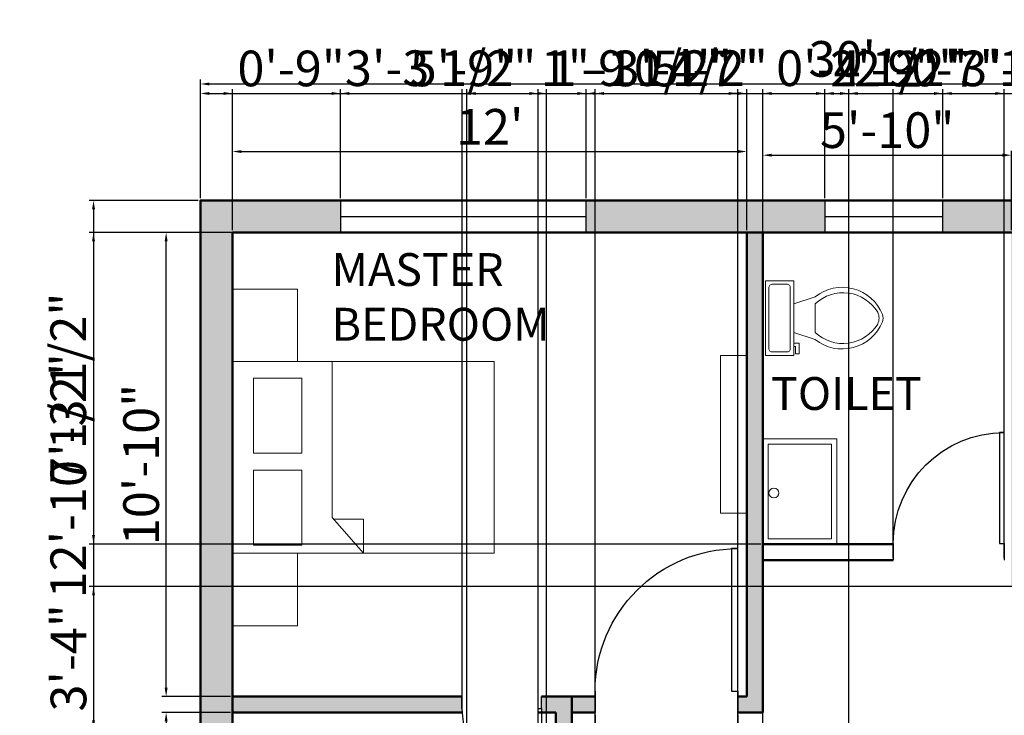
# Model space of a CAD drawing. Units: inches. Extents: x 1344 to 2521, y 3236 to 4924.
# Tile 6 of 14: x 1968 to 2244, y 3619 to 3814. Entities that reach past the tile are written whole.
import ezdxf

# ---------------------------------------------------------------- set-up
doc = ezdxf.new("R2010")
doc.units = ezdxf.units.IN
for name, color, linetype, lineweight in [('A-ANNO-DIMS', 2, 'Continuous', 18), ('A-AREA-IDEN', 3, 'Continuous', 18), ('A-DOOR', 50, 'Continuous', 25), ('A-FLOR-FIXT', 8, 'Continuous', 18), ('A-FURN', 130, 'Continuous', 18), ('A-GLAZ', 150, 'Continuous', 25), ('A-WALL', 31, 'Continuous', 50), ('A-WALL-PATT', 8, 'Continuous', 13)]:
    doc.layers.add(name, color=color, linetype=linetype, lineweight=lineweight)
doc.styles.get("Standard").update_dxf_attribs({"font": 'arial.ttf'})
doc.dimstyles.new('ISO-25', dxfattribs={"dimtxt": 10, "dimasz": 2.5, "dimexe": 1.25, "dimexo": 0.625, "dimtad": 1, "dimdec": 0, "dimlunit": 4, "dimtxsty": 'Standard', "dimcen": 2.5, "dimadec": 0, "dimazin": 0, "dimtfac": 1, "dimtdec": 0, "dimtmove": 0, "dimatfit": 3, "dimfxl": 1, "dimarcsym": 0})

# ---------------------------------------------------------------- blocks, each defined once
blk = doc.blocks.new('*U2')
for p, q in [((0, 0), (0, -6)), ((40, 0), (40, -6))]:
    blk.add_line(p, q)
blk.add_lwpolyline([(0, 0), (0, 40), (1.75, 40), (1.75, 0)], close=True)
blk.add_arc((0, 0), 40, 0, 90)
blk = doc.blocks.new('*U6')
for p, q in [((9.5, -6), (9.5, -2)), ((-8, -8.5), (-8, -8)), ((-7, -8), (-7, -9.5)), ((-4, -8), (-6, -14)), ((4, -8), (6, -14)), ((-10, -8.5), (-8, -8.5)), ((-10, -9.5), (-10, -8.5)), ((-7, -9.5), (-10, -9.5)), ((4, -14), (-4, -14))]:
    blk.add_line(p, q)
blk.add_lwpolyline([(10.5, -8), (10.5, 0), (-10.5, 0), (-10.5, -8)], close=True)
for points in [[(-9.5, -2), (-9.5, -6)], [(8.5, -1), (-8.5, -1)], [(-8.5, -7), (8.5, -7)]]:
    blk.add_lwpolyline(points)
for centre, radius, start, end in [((-8.62, -1.88), 0.884, 81.8699, 188.1301), ((8.62, -1.88), 0.884, 351.8699, 98.1301), ((-8.62, -6.12), 0.884, 171.8699, 278.1301), ((8.62, -6.12), 0.884, 261.8699, 8.1301), ((3.52, -21.58), 12.17, 141.4691, 247.9714), ((4.2, -21.82), 11.33, 136.3677, 238.9468), ((-3.52, -21.58), 12.17, 292.0284, 38.5307), ((-4.2, -21.82), 11.33, 301.053, 43.6321), ((0, -27.88), 4, 245.7318, 294.2682), ((0, -29), 4, 254.8605, 285.1395)]:
    blk.add_arc(centre, radius, start, end)
blk = doc.blocks.new('*D47')
at = {"layer": 'A-ANNO-DIMS', "color": 0, "lineweight": -2, "transparency": 16777216}
for p, q in [((2018.36, 3764.06), (2018.36, 3797.35)), ((2378.36, 3764.06), (2378.36, 3797.35)), ((2020.86, 3796.1), (2375.86, 3796.1))]:
    blk.add_line(p, q, dxfattribs=at)
at = {"layer": 'A-ANNO-DIMS', "color": 0, "lineweight": 100, "transparency": 16777216}
for points in [[(2020.86, 3796.52), (2020.86, 3795.69), (2018.36, 3796.1)], [(2375.86, 3796.52), (2375.86, 3795.69), (2378.36, 3796.1)]]:
    blk.add_solid(points, dxfattribs=at)
at = {"layer": 'Defpoints', "color": 0, "lineweight": 100, "transparency": 16777216}
for p in [(2378.36, 3796.1), (2018.36, 3763.43), (2378.36, 3763.43)]:
    blk.add_point(p, dxfattribs=at)
at = {"layer": 'A-ANNO-DIMS', "color": 0, "transparency": 16777216, "insert": (2198.36, 3801.84), "char_height": 10, "attachment_point": 5}
blk.add_mtext("30'", dxfattribs=at)
blk = doc.blocks.new('*D48')
at = {"layer": 'A-ANNO-DIMS', "color": 0, "lineweight": -2, "transparency": 16777216}
for p, q in [((2027.36, 3755.06), (2027.36, 3778.39)), ((2171.6, 3755.06), (2171.6, 3778.39)), ((2029.86, 3777.14), (2169.1, 3777.14))]:
    blk.add_line(p, q, dxfattribs=at)
at = {"layer": 'A-ANNO-DIMS', "color": 0, "lineweight": 100, "transparency": 16777216}
for points in [[(2029.86, 3777.55), (2029.86, 3776.72), (2027.36, 3777.14)], [(2169.1, 3777.55), (2169.1, 3776.72), (2171.6, 3777.14)]]:
    blk.add_solid(points, dxfattribs=at)
at = {"layer": 'Defpoints', "color": 0, "lineweight": 100, "transparency": 16777216}
for p in [(2171.6, 3777.14), (2027.36, 3754.43), (2171.6, 3754.43)]:
    blk.add_point(p, dxfattribs=at)
at = {"layer": 'A-ANNO-DIMS', "color": 0, "transparency": 16777216, "insert": (2099.48, 3782.78), "char_height": 10, "attachment_point": 5}
blk.add_mtext("12'", dxfattribs=at)
blk = doc.blocks.new('*D49')
at = {"layer": 'A-ANNO-DIMS', "color": 0, "lineweight": -2, "transparency": 16777216}
for p, q in [((2176.1, 3755.06), (2176.1, 3777.36)), ((2178.6, 3776.11), (2243.29, 3776.11)), ((2245.79, 3755.06), (2245.79, 3777.36))]:
    blk.add_line(p, q, dxfattribs=at)
at = {"layer": 'A-ANNO-DIMS', "color": 0, "lineweight": 100, "transparency": 16777216}
for points in [[(2178.6, 3776.53), (2178.6, 3775.69), (2176.1, 3776.11)], [(2243.29, 3776.53), (2243.29, 3775.69), (2245.79, 3776.11)]]:
    blk.add_solid(points, dxfattribs=at)
at = {"layer": 'Defpoints', "color": 0, "lineweight": 100, "transparency": 16777216}
for p in [(2245.79, 3776.11), (2176.1, 3754.43), (2245.79, 3754.43)]:
    blk.add_point(p, dxfattribs=at)
at = {"layer": 'A-ANNO-DIMS', "color": 0, "transparency": 16777216, "insert": (2210.94, 3781.84), "char_height": 10, "attachment_point": 5}
blk.add_mtext('5\'-10"', dxfattribs=at)
blk = doc.blocks.new('*D51')
at = {"layer": 'A-ANNO-DIMS', "color": 0, "lineweight": -2, "transparency": 16777216}
for p, q in [((2026.74, 3754.43), (2007.48, 3754.43)), ((2008.73, 3626.69), (2008.73, 3751.93)), ((2026.74, 3624.19), (2007.48, 3624.19))]:
    blk.add_line(p, q, dxfattribs=at)
at = {"layer": 'A-ANNO-DIMS', "color": 0, "lineweight": 100, "transparency": 16777216}
for points in [[(2008.31, 3751.93), (2009.14, 3751.93), (2008.73, 3754.43)], [(2008.31, 3626.69), (2009.14, 3626.69), (2008.73, 3624.19)]]:
    blk.add_solid(points, dxfattribs=at)
at = {"layer": 'Defpoints', "color": 0, "lineweight": 100, "transparency": 16777216}
for p in [(2008.73, 3754.43), (2027.36, 3754.43), (2027.36, 3624.19)]:
    blk.add_point(p, dxfattribs=at)
at = {"layer": 'A-ANNO-DIMS', "color": 0, "transparency": 16777216, "insert": (2003, 3689.31), "char_height": 10, "attachment_point": 5, "rotation": 90}
blk.add_mtext('10\'-10"', dxfattribs=at)
blk = doc.blocks.new('*D52')
at = {"layer": 'A-ANNO-DIMS', "color": 0, "lineweight": -2, "transparency": 16777216}
for p, q in [((2026.74, 3619.69), (2007.48, 3619.69)), ((2008.73, 3617.19), (2008.73, 3575.82)), ((2026.74, 3573.32), (2007.48, 3573.32))]:
    blk.add_line(p, q, dxfattribs=at)
at = {"layer": 'A-ANNO-DIMS', "color": 0, "lineweight": 100, "transparency": 16777216}
for points in [[(2008.31, 3617.19), (2009.14, 3617.19), (2008.73, 3619.69)], [(2008.31, 3575.82), (2009.14, 3575.82), (2008.73, 3573.32)]]:
    blk.add_solid(points, dxfattribs=at)
at = {"layer": 'Defpoints', "color": 0, "lineweight": 100, "transparency": 16777216}
for p in [(2027.36, 3619.69), (2008.73, 3573.32), (2027.36, 3573.32)]:
    blk.add_point(p, dxfattribs=at)
at = {"layer": 'A-ANNO-DIMS', "color": 0, "transparency": 16777216, "insert": (2002.99, 3596.5), "char_height": 10, "attachment_point": 5, "rotation": 90}
blk.add_mtext('3\'-10"', dxfattribs=at)
blk = doc.blocks.new('BED-DOUBLE')
for p, q in [((27.95, 53.78), (27.95, 9.98)), ((27.95, 9.98), (36.68, 0)), ((36.68, 9.56), (28.32, 9.56)), ((36.68, 0), (36.68, 9.56))]:
    blk.add_line(p, q)
for points in [[(0, 0), (73.35, 0), (73.35, 53.78), (0, 53.78)], [(5.91, 28.08), (19.39, 28.08), (19.39, 49.13), (5.91, 49.13)], [(5.91, 2.27), (19.39, 2.27), (19.39, 23.31), (5.91, 23.31)]]:
    blk.add_lwpolyline(points, close=True)
blk = doc.blocks.new('WASH-BASIN')
for points in [[(29.51, 20.73), (0, 20.73), (0, 0), (29.51, 0)], [(28.05, 19.27), (1.46, 19.27), (1.46, 1.46), (28.05, 1.46)]]:
    blk.add_lwpolyline(points, close=True)
blk.add_circle((14.31, 17.66), 1.38)
blk = doc.blocks.new('*D186')
at = {"layer": 'A-ANNO-DIMS', "color": 0, "lineweight": -2, "transparency": 16777216}
for p, q in [((2017.74, 3763.43), (1987.11, 3763.43)), ((1988.36, 3760.93), (1988.36, 3350.01)), ((2017.74, 3347.51), (1987.11, 3347.51))]:
    blk.add_line(p, q, dxfattribs=at)
at = {"layer": 'A-ANNO-DIMS', "color": 0, "lineweight": 100, "transparency": 16777216}
for points in [[(1987.95, 3760.93), (1988.78, 3760.93), (1988.36, 3763.43)], [(1987.95, 3350.01), (1988.78, 3350.01), (1988.36, 3347.51)]]:
    blk.add_solid(points, dxfattribs=at)
at = {"layer": 'Defpoints', "color": 0, "lineweight": 100, "transparency": 16777216}
for p in [(2018.36, 3763.43), (1988.36, 3347.51), (2018.36, 3347.51)]:
    blk.add_point(p, dxfattribs=at)
at = {"layer": 'A-ANNO-DIMS', "color": 0, "transparency": 16777216, "insert": (1982.63, 3555.47), "char_height": 10, "attachment_point": 5, "rotation": 90}
blk.add_mtext('34\'-8"', dxfattribs=at)
blk = doc.blocks.new('*D187')
at = {"layer": 'A-ANNO-DIMS', "color": 0, "lineweight": -2, "transparency": 16777216}
for p, q in [((2018.36, 3764.06), (2018.36, 3794.68)), ((2027.36, 3755.06), (2027.36, 3794.68)), ((2020.86, 3793.43), (2024.86, 3793.43)), ((2027.36, 3793.43), (2057.7, 3793.43))]:
    blk.add_line(p, q, dxfattribs=at)
at = {"layer": 'A-ANNO-DIMS', "color": 0, "lineweight": 100, "transparency": 16777216}
for points in [[(2020.86, 3793.85), (2020.86, 3793.02), (2018.36, 3793.43)], [(2024.86, 3793.85), (2024.86, 3793.02), (2027.36, 3793.43)]]:
    blk.add_solid(points, dxfattribs=at)
at = {"layer": 'Defpoints', "color": 0, "lineweight": 100, "transparency": 16777216}
for p in [(2027.36, 3793.43), (2018.36, 3763.43), (2027.36, 3754.43)]:
    blk.add_point(p, dxfattribs=at)
at = {"layer": 'A-ANNO-DIMS', "color": 0, "transparency": 16777216, "insert": (2043.78, 3799.16), "char_height": 10, "attachment_point": 5}
blk.add_mtext('0\'-9"', dxfattribs=at)
blk = doc.blocks.new('*D188')
at = {"layer": 'A-ANNO-DIMS', "color": 0, "lineweight": -2, "transparency": 16777216}
for p, q in [((2171.6, 3755.06), (2171.6, 3794.68)), ((2176.1, 3755.06), (2176.1, 3794.68)), ((2169.1, 3793.43), (2166.6, 3793.43)), ((2171.6, 3793.43), (2176.1, 3793.43)), ((2178.6, 3793.43), (2232.23, 3793.43))]:
    blk.add_line(p, q, dxfattribs=at)
at = {"layer": 'A-ANNO-DIMS', "color": 0, "lineweight": 100, "transparency": 16777216}
for points in [[(2169.1, 3793.85), (2169.1, 3793.02), (2171.6, 3793.43)], [(2178.6, 3793.85), (2178.6, 3793.02), (2176.1, 3793.43)]]:
    blk.add_solid(points, dxfattribs=at)
at = {"layer": 'Defpoints', "color": 0, "lineweight": 100, "transparency": 16777216}
for p in [(2176.1, 3793.43), (2171.6, 3754.43), (2176.1, 3754.43)]:
    blk.add_point(p, dxfattribs=at)
at = {"layer": 'A-ANNO-DIMS', "color": 0, "transparency": 16777216, "insert": (2206.66, 3799.23), "char_height": 10, "attachment_point": 5}
blk.add_mtext('0\'-4 1/2"', dxfattribs=at)
blk = doc.blocks.new('*D189')
at = {"layer": 'A-ANNO-DIMS', "color": 0, "lineweight": -2, "transparency": 16777216}
for p, q in [((2018.36, 3764.06), (2018.36, 3794.68)), ((2057.65, 3764.06), (2057.65, 3794.68)), ((2020.86, 3793.43), (2055.15, 3793.43)), ((2057.65, 3793.43), (2111.27, 3793.43))]:
    blk.add_line(p, q, dxfattribs=at)
at = {"layer": 'A-ANNO-DIMS', "color": 0, "lineweight": 100, "transparency": 16777216}
for points in [[(2020.86, 3793.85), (2020.86, 3793.02), (2018.36, 3793.43)], [(2055.15, 3793.85), (2055.15, 3793.02), (2057.65, 3793.43)]]:
    blk.add_solid(points, dxfattribs=at)
at = {"layer": 'Defpoints', "color": 0, "lineweight": 100, "transparency": 16777216}
for p in [(2057.65, 3793.43), (2018.36, 3763.43), (2057.65, 3763.43)]:
    blk.add_point(p, dxfattribs=at)
at = {"layer": 'A-ANNO-DIMS', "color": 0, "transparency": 16777216, "insert": (2085.71, 3799.23), "char_height": 10, "attachment_point": 5}
blk.add_mtext('3\'-3 1/2"', dxfattribs=at)
blk = doc.blocks.new('*D190')
at = {"layer": 'A-ANNO-DIMS', "color": 0, "lineweight": -2, "transparency": 16777216}
for p, q in [((2057.65, 3764.06), (2057.65, 3794.68)), ((2126.57, 3764.06), (2126.57, 3794.68)), ((2060.15, 3793.43), (2124.07, 3793.43))]:
    blk.add_line(p, q, dxfattribs=at)
at = {"layer": 'A-ANNO-DIMS', "color": 0, "lineweight": 100, "transparency": 16777216}
for points in [[(2060.15, 3793.85), (2060.15, 3793.02), (2057.65, 3793.43)], [(2124.07, 3793.85), (2124.07, 3793.02), (2126.57, 3793.43)]]:
    blk.add_solid(points, dxfattribs=at)
at = {"layer": 'Defpoints', "color": 0, "lineweight": 100, "transparency": 16777216}
for p in [(2126.57, 3793.43), (2057.65, 3763.43), (2126.57, 3763.43)]:
    blk.add_point(p, dxfattribs=at)
at = {"layer": 'A-ANNO-DIMS', "color": 0, "transparency": 16777216, "insert": (2092.11, 3799.16), "char_height": 10, "attachment_point": 5}
blk.add_mtext('5\'-9"', dxfattribs=at)
blk = doc.blocks.new('*D191')
at = {"layer": 'A-ANNO-DIMS', "color": 0, "lineweight": -2, "transparency": 16777216}
for p, q in [((2126.57, 3764.06), (2126.57, 3794.68)), ((2193.45, 3764.06), (2193.45, 3794.68)), ((2129.07, 3793.43), (2190.95, 3793.43))]:
    blk.add_line(p, q, dxfattribs=at)
at = {"layer": 'A-ANNO-DIMS', "color": 0, "lineweight": 100, "transparency": 16777216}
for points in [[(2129.07, 3793.85), (2129.07, 3793.02), (2126.57, 3793.43)], [(2190.95, 3793.85), (2190.95, 3793.02), (2193.45, 3793.43)]]:
    blk.add_solid(points, dxfattribs=at)
at = {"layer": 'Defpoints', "color": 0, "lineweight": 100, "transparency": 16777216}
for p in [(2193.45, 3793.43), (2126.57, 3763.43), (2193.45, 3763.43)]:
    blk.add_point(p, dxfattribs=at)
at = {"layer": 'A-ANNO-DIMS', "color": 0, "transparency": 16777216, "insert": (2160.01, 3799.14), "char_height": 10, "attachment_point": 5}
blk.add_mtext('5\'-7"', dxfattribs=at)
blk = doc.blocks.new('*D192')
at = {"layer": 'A-ANNO-DIMS', "color": 0, "lineweight": -2, "transparency": 16777216}
for p, q in [((2193.45, 3764.06), (2193.45, 3794.68)), ((2226.56, 3764.06), (2226.56, 3794.68)), ((2195.95, 3793.43), (2224.06, 3793.43))]:
    blk.add_line(p, q, dxfattribs=at)
at = {"layer": 'A-ANNO-DIMS', "color": 0, "lineweight": 100, "transparency": 16777216}
for points in [[(2195.95, 3793.85), (2195.95, 3793.02), (2193.45, 3793.43)], [(2224.06, 3793.85), (2224.06, 3793.02), (2226.56, 3793.43)]]:
    blk.add_solid(points, dxfattribs=at)
at = {"layer": 'Defpoints', "color": 0, "lineweight": 100, "transparency": 16777216}
for p in [(2226.56, 3793.43), (2193.45, 3763.43), (2226.56, 3763.43)]:
    blk.add_point(p, dxfattribs=at)
at = {"layer": 'A-ANNO-DIMS', "color": 0, "transparency": 16777216, "insert": (2210.01, 3799.16), "char_height": 10, "attachment_point": 5}
blk.add_mtext('2\'-9"', dxfattribs=at)
blk = doc.blocks.new('*D193')
at = {"layer": 'A-ANNO-DIMS', "color": 0, "lineweight": -2, "transparency": 16777216}
for p, q in [((2226.56, 3764.06), (2226.56, 3794.68)), ((2266.48, 3764.06), (2266.48, 3794.68)), ((2229.06, 3793.43), (2263.98, 3793.43))]:
    blk.add_line(p, q, dxfattribs=at)
at = {"layer": 'A-ANNO-DIMS', "color": 0, "lineweight": 100, "transparency": 16777216}
for points in [[(2229.06, 3793.85), (2229.06, 3793.02), (2226.56, 3793.43)], [(2263.98, 3793.85), (2263.98, 3793.02), (2266.48, 3793.43)]]:
    blk.add_solid(points, dxfattribs=at)
at = {"layer": 'Defpoints', "color": 0, "lineweight": 100, "transparency": 16777216}
for p in [(2266.48, 3793.43), (2226.56, 3763.43), (2266.48, 3763.43)]:
    blk.add_point(p, dxfattribs=at)
at = {"layer": 'A-ANNO-DIMS', "color": 0, "transparency": 16777216, "insert": (2246.52, 3799.17), "char_height": 10, "attachment_point": 5}
blk.add_mtext('3\'-4"', dxfattribs=at)
blk = doc.blocks.new('*D196')
at = {"layer": 'A-ANNO-DIMS', "color": 0, "lineweight": -2, "transparency": 16777216}
for p, q in [((2017.74, 3763.43), (1987.11, 3763.43)), ((1988.36, 3760.93), (1988.36, 3611.37)), ((2017.74, 3608.87), (1987.11, 3608.87))]:
    blk.add_line(p, q, dxfattribs=at)
at = {"layer": 'A-ANNO-DIMS', "color": 0, "lineweight": 100, "transparency": 16777216}
for points in [[(1987.95, 3760.93), (1988.78, 3760.93), (1988.36, 3763.43)], [(1987.95, 3611.37), (1988.78, 3611.37), (1988.36, 3608.87)]]:
    blk.add_solid(points, dxfattribs=at)
at = {"layer": 'Defpoints', "color": 0, "lineweight": 100, "transparency": 16777216}
for p in [(2018.36, 3763.43), (1988.36, 3608.87), (2018.36, 3608.87)]:
    blk.add_point(p, dxfattribs=at)
at = {"layer": 'A-ANNO-DIMS', "color": 0, "transparency": 16777216, "insert": (1982.57, 3686.15), "char_height": 10, "attachment_point": 5, "rotation": 90}
blk.add_mtext('12\'-10 1/2"', dxfattribs=at)
blk = doc.blocks.new('*D208')
at = {"layer": 'A-ANNO-DIMS', "color": 0, "lineweight": -2, "transparency": 16777216}
for p, q in [((2091.72, 3620.31), (2091.72, 3794.68)), ((2113.05, 3620.31), (2113.05, 3794.68)), ((2094.22, 3793.43), (2110.55, 3793.43)), ((2113.05, 3793.43), (2165.74, 3793.43))]:
    blk.add_line(p, q, dxfattribs=at)
at = {"layer": 'A-ANNO-DIMS', "color": 0, "lineweight": 100, "transparency": 16777216}
for points in [[(2094.22, 3793.85), (2094.22, 3793.02), (2091.72, 3793.43)], [(2110.55, 3793.85), (2110.55, 3793.02), (2113.05, 3793.43)]]:
    blk.add_solid(points, dxfattribs=at)
at = {"layer": 'Defpoints', "color": 0, "lineweight": 100, "transparency": 16777216}
for p in [(2113.05, 3793.43), (2091.72, 3619.69), (2113.05, 3619.69)]:
    blk.add_point(p, dxfattribs=at)
at = {"layer": 'A-ANNO-DIMS', "color": 0, "transparency": 16777216, "insert": (2140.64, 3799.23), "char_height": 10, "attachment_point": 5}
blk.add_mtext('1\'-9 1/2"', dxfattribs=at)
blk = doc.blocks.new('*D209')
at = {"layer": 'A-ANNO-DIMS', "color": 0, "lineweight": -2, "transparency": 16777216}
for p, q in [((2129.02, 3619.06), (2129.02, 3316.22)), ((2169.02, 3619.06), (2169.02, 3316.22)), ((2131.52, 3317.47), (2166.52, 3317.47))]:
    blk.add_line(p, q, dxfattribs=at)
at = {"layer": 'A-ANNO-DIMS', "color": 0, "lineweight": 100, "transparency": 16777216}
for points in [[(2131.52, 3317.89), (2131.52, 3317.06), (2129.02, 3317.47)], [(2166.52, 3317.89), (2166.52, 3317.06), (2169.02, 3317.47)]]:
    blk.add_solid(points, dxfattribs=at)
at = {"layer": 'Defpoints', "color": 0, "lineweight": 100, "transparency": 16777216}
for p in [(2129.02, 3619.69), (2169.02, 3619.69), (2169.02, 3317.47)]:
    blk.add_point(p, dxfattribs=at)
at = {"layer": 'A-ANNO-DIMS', "color": 0, "transparency": 16777216, "insert": (2149.02, 3323.21), "char_height": 10, "attachment_point": 5}
blk.add_mtext('3\'-4"', dxfattribs=at)
blk = doc.blocks.new('*D210')
at = {"layer": 'A-ANNO-DIMS', "color": 0, "lineweight": -2, "transparency": 16777216}
for p, q in [((2093.06, 3515.07), (2093.06, 3794.68)), ((2115.39, 3515.07), (2115.39, 3794.68)), ((2095.56, 3793.43), (2112.89, 3793.43)), ((2115.39, 3793.43), (2175.85, 3793.43))]:
    blk.add_line(p, q, dxfattribs=at)
at = {"layer": 'A-ANNO-DIMS', "color": 0, "lineweight": 100, "transparency": 16777216}
for points in [[(2095.56, 3793.85), (2095.56, 3793.02), (2093.06, 3793.43)], [(2112.89, 3793.85), (2112.89, 3793.02), (2115.39, 3793.43)]]:
    blk.add_solid(points, dxfattribs=at)
at = {"layer": 'Defpoints', "color": 0, "lineweight": 100, "transparency": 16777216}
for p in [(2115.39, 3793.43), (2093.06, 3514.45), (2115.39, 3514.45)]:
    blk.add_point(p, dxfattribs=at)
at = {"layer": 'A-ANNO-DIMS', "color": 0, "transparency": 16777216, "insert": (2146.87, 3799.23), "char_height": 10, "attachment_point": 5}
blk.add_mtext('1\'-10 1/2"', dxfattribs=at)
blk = doc.blocks.new('*D211')
at = {"layer": 'A-ANNO-DIMS', "color": 0, "lineweight": -2, "transparency": 16777216}
for p, q in [((2129.02, 3519.57), (2129.02, 3794.68)), ((2169.02, 3519.57), (2169.02, 3794.68)), ((2131.52, 3793.43), (2166.52, 3793.43))]:
    blk.add_line(p, q, dxfattribs=at)
at = {"layer": 'A-ANNO-DIMS', "color": 0, "lineweight": 100, "transparency": 16777216}
for points in [[(2131.52, 3793.85), (2131.52, 3793.02), (2129.02, 3793.43)], [(2166.52, 3793.85), (2166.52, 3793.02), (2169.02, 3793.43)]]:
    blk.add_solid(points, dxfattribs=at)
at = {"layer": 'Defpoints', "color": 0, "lineweight": 100, "transparency": 16777216}
for p in [(2169.02, 3793.43), (2129.02, 3518.95), (2169.02, 3518.95)]:
    blk.add_point(p, dxfattribs=at)
at = {"layer": 'A-ANNO-DIMS', "color": 0, "transparency": 16777216, "insert": (2149.02, 3799.17), "char_height": 10, "attachment_point": 5}
blk.add_mtext('3\'-4"', dxfattribs=at)
blk = doc.blocks.new('*D212')
at = {"layer": 'A-ANNO-DIMS', "color": 0, "lineweight": -2, "transparency": 16777216}
for p, q in [((2175.47, 3754.43), (1987.11, 3754.43)), ((1988.36, 3751.93), (1988.36, 3669.49)), ((2175.47, 3666.99), (1987.11, 3666.99))]:
    blk.add_line(p, q, dxfattribs=at)
at = {"layer": 'A-ANNO-DIMS', "color": 0, "lineweight": 100, "transparency": 16777216}
for points in [[(1987.95, 3751.93), (1988.78, 3751.93), (1988.36, 3754.43)], [(1987.95, 3669.49), (1988.78, 3669.49), (1988.36, 3666.99)]]:
    blk.add_solid(points, dxfattribs=at)
at = {"layer": 'Defpoints', "color": 0, "lineweight": 100, "transparency": 16777216}
for p in [(2176.1, 3754.43), (1988.36, 3666.99), (2176.1, 3666.99)]:
    blk.add_point(p, dxfattribs=at)
at = {"layer": 'A-ANNO-DIMS', "color": 0, "transparency": 16777216, "insert": (1982.56, 3710.71), "char_height": 10, "attachment_point": 5, "rotation": 90}
blk.add_mtext('7\'-3 1/2"', dxfattribs=at)
blk = doc.blocks.new('*D213')
at = {"layer": 'A-ANNO-DIMS', "color": 0, "lineweight": -2, "transparency": 16777216}
for p, q in [((2212.67, 3663.12), (2212.67, 3794.68)), ((2243.8, 3663.12), (2243.8, 3794.68)), ((2215.17, 3793.43), (2241.3, 3793.43))]:
    blk.add_line(p, q, dxfattribs=at)
at = {"layer": 'A-ANNO-DIMS', "color": 0, "lineweight": 100, "transparency": 16777216}
for points in [[(2215.17, 3793.85), (2215.17, 3793.02), (2212.67, 3793.43)], [(2241.3, 3793.85), (2241.3, 3793.02), (2243.8, 3793.43)]]:
    blk.add_solid(points, dxfattribs=at)
at = {"layer": 'Defpoints', "color": 0, "lineweight": 100, "transparency": 16777216}
for p in [(2243.8, 3793.43), (2212.67, 3662.49), (2243.8, 3662.49)]:
    blk.add_point(p, dxfattribs=at)
at = {"layer": 'A-ANNO-DIMS', "color": 0, "transparency": 16777216, "insert": (2228.24, 3799.08), "char_height": 10, "attachment_point": 5}
blk.add_mtext('2\'-7"', dxfattribs=at)
blk = doc.blocks.new('*D214')
at = {"layer": 'A-ANNO-DIMS', "color": 0, "lineweight": -2, "transparency": 16777216}
for p, q in [((2249.66, 3655.04), (1987.11, 3655.04)), ((1988.36, 3652.54), (1988.36, 3617.54)), ((2249.66, 3615.04), (1987.11, 3615.04))]:
    blk.add_line(p, q, dxfattribs=at)
at = {"layer": 'A-ANNO-DIMS', "color": 0, "lineweight": 100, "transparency": 16777216}
for points in [[(1987.95, 3652.54), (1988.78, 3652.54), (1988.36, 3655.04)], [(1987.95, 3617.54), (1988.78, 3617.54), (1988.36, 3615.04)]]:
    blk.add_solid(points, dxfattribs=at)
at = {"layer": 'Defpoints', "color": 0, "lineweight": 100, "transparency": 16777216}
for p in [(2250.29, 3655.04), (1988.36, 3615.04), (2250.29, 3615.04)]:
    blk.add_point(p, dxfattribs=at)
at = {"layer": 'A-ANNO-DIMS', "color": 0, "transparency": 16777216, "insert": (1982.63, 3635.04), "char_height": 10, "attachment_point": 5, "rotation": 90}
blk.add_mtext('3\'-4"', dxfattribs=at)
blk = doc.blocks.new('*D216')
at = {"layer": 'A-ANNO-DIMS', "color": 0, "lineweight": -2, "transparency": 16777216}
for p, q in [((2176.1, 3403.64), (2176.1, 3794.68)), ((2200.2, 3403.64), (2200.2, 3794.68)), ((2178.6, 3793.43), (2197.7, 3793.43)), ((2200.2, 3793.43), (2230.7, 3793.43))]:
    blk.add_line(p, q, dxfattribs=at)
at = {"layer": 'A-ANNO-DIMS', "color": 0, "lineweight": 100, "transparency": 16777216}
for points in [[(2178.6, 3793.85), (2178.6, 3793.02), (2176.1, 3793.43)], [(2197.7, 3793.85), (2197.7, 3793.02), (2200.2, 3793.43)]]:
    blk.add_solid(points, dxfattribs=at)
at = {"layer": 'Defpoints', "color": 0, "lineweight": 100, "transparency": 16777216}
for p in [(2200.2, 3793.43), (2176.1, 3403.01), (2200.2, 3403.01)]:
    blk.add_point(p, dxfattribs=at)
at = {"layer": 'A-ANNO-DIMS', "color": 0, "transparency": 16777216, "insert": (2216.7, 3799.16), "char_height": 10, "attachment_point": 5}
blk.add_mtext('2\'-0"', dxfattribs=at)
blk = doc.blocks.new('*D217')
at = {"layer": 'A-ANNO-DIMS', "color": 0, "lineweight": -2, "transparency": 16777216}
for p, q in [((2200.2, 3403.64), (2200.2, 3794.68)), ((2345.46, 3403.64), (2345.46, 3794.68)), ((2202.7, 3793.43), (2342.96, 3793.43))]:
    blk.add_line(p, q, dxfattribs=at)
at = {"layer": 'A-ANNO-DIMS', "color": 0, "lineweight": 100, "transparency": 16777216}
for points in [[(2202.7, 3793.85), (2202.7, 3793.02), (2200.2, 3793.43)], [(2342.96, 3793.85), (2342.96, 3793.02), (2345.46, 3793.43)]]:
    blk.add_solid(points, dxfattribs=at)
at = {"layer": 'Defpoints', "color": 0, "lineweight": 100, "transparency": 16777216}
for p in [(2345.46, 3793.43), (2200.2, 3403.01), (2345.46, 3403.01)]:
    blk.add_point(p, dxfattribs=at)
at = {"layer": 'A-ANNO-DIMS', "color": 0, "transparency": 16777216, "insert": (2272.83, 3799.23), "char_height": 10, "attachment_point": 5}
blk.add_mtext('12\'-1 1/2"', dxfattribs=at)

msp = doc.modelspace()

# ---------------------------------------------------------------- hatches: boundary and pattern name
at = {"layer": 'A-WALL-PATT'}
h = msp.add_hatch(color=256, dxfattribs=at)
h.dxf.hatch_style = 1
h.paths.add_polyline_path([(2193.45, 3763.43), (2126.57, 3763.43), (2126.57, 3754.43), (2193.45, 3754.43)])
h.paths.add_polyline_path([(2057.65, 3763.43), (2018.36, 3763.43), (2018.36, 3608.87), (2027.36, 3608.87), (2027.36, 3754.43), (2057.65, 3754.43)])
h.paths.add_polyline_path([(2266.48, 3763.43), (2226.56, 3763.43), (2226.56, 3754.43), (2266.48, 3754.43)])
h.paths.add_polyline_path([(2378.36, 3763.43), (2335.41, 3763.43), (2335.41, 3754.43), (2369.36, 3754.43), (2369.36, 3594.28), (2378.36, 3594.28)])
h.paths.add_polyline_path([(2369.36, 3610.02), (2250.29, 3610.02), (2250.29, 3605.52), (2369.36, 3605.52)])
h.paths.add_polyline_path([(2250.29, 3610.02), (2245.79, 3610.02), (2245.79, 3605.52), (2250.29, 3605.52)])
h.paths.add_polyline_path([(2250.29, 3754.43), (2245.79, 3754.43), (2245.79, 3655.04), (2250.29, 3655.04)])
h.paths.add_polyline_path([(2176.1, 3754.43), (2171.6, 3754.43), (2171.6, 3624.19), (2171.35, 3624.19), (2169.02, 3624.19), (2169.02, 3619.69), (2176.1, 3619.69)])
h.paths.add_polyline_path([(2129.02, 3624.19), (2122.52, 3624.19), (2122.52, 3619.69), (2129.02, 3619.69)])
h.paths.add_polyline_path([(2091.69, 3624.19), (2027.36, 3624.19), (2027.36, 3619.69), (2091.72, 3619.69, -0.012876), (2091.69, 3620.84)])
h.paths.add_polyline_path([(2250.29, 3615.04), (2245.79, 3615.04), (2245.79, 3610.02), (2250.29, 3610.02)])
h.paths.add_polyline_path([(2027.36, 3580.89), (2018.36, 3580.89), (2018.36, 3555.45), (2027.36, 3555.45)])
h.paths.add_polyline_path([(2027.36, 3527.47), (2018.36, 3527.47), (2018.36, 3455.82), (2027.36, 3455.82)])
h.paths.add_polyline_path([(2093.06, 3517.8, -0.012876), (2093.09, 3518.95), (2027.36, 3518.95), (2027.36, 3514.45), (2093.06, 3514.45)])
h.paths.add_polyline_path([(2118.02, 3573.32), (2110.02, 3573.32), (2110.02, 3573.28), (2080.51, 3573.28), (2027.36, 3573.32), (2027.36, 3568.82), (2118.02, 3568.82)])
h.paths.add_polyline_path([(2122.52, 3624.19), (2114.02, 3624.19), (2114.02, 3620.84), (2114.02, 3619.69), (2118.02, 3619.69), (2118.02, 3518.95), (2122.52, 3518.95)])
h.paths.add_polyline_path([(2129.02, 3518.95), (2115.39, 3518.95), (2115.39, 3517.8), (2115.39, 3514.45), (2129.02, 3514.45)])
h.paths.add_polyline_path([(2027.36, 3386.9), (2018.36, 3386.9), (2018.36, 3347.51), (2056.7, 3347.51), (2056.7, 3356.47), (2027.36, 3356.47)])
h.paths.add_polyline_path([(2187.76, 3356.47), (2168.81, 3356.47), (2149.67, 3356.47), (2125.62, 3356.47), (2125.62, 3347.51), (2176.1, 3347.51), (2187.76, 3347.51)])
h.paths.add_polyline_path([(2378.36, 3525.36), (2369.36, 3525.36), (2369.36, 3497.27), (2369.36, 3412.01), (2369.57, 3412.01), (2369.57, 3403.01), (2369.36, 3356.51), (2369.36, 3347.51), (2378.36, 3347.51)])
h.paths.add_polyline_path([(2369.36, 3412.01), (2345.46, 3412.01), (2345.46, 3403.01), (2369.36, 3403.01)])
h.paths.add_polyline_path([(2206.56, 3518.95), (2176.1, 3518.95), (2176.1, 3514.45), (2206.56, 3514.45)])
h.paths.add_polyline_path([(2130.92, 3560.64), (2239.92, 3560.64), (2239.92, 3579.62), (2130.92, 3579.62)], flags=9)
h.paths.add_polyline_path([(2271.24, 3730.09), (2345.91, 3730.09), (2345.91, 3749.07), (2271.24, 3749.07)], flags=9)
h.paths.add_polyline_path([(2051.28, 3467.76), (2122.39, 3467.76), (2122.39, 3502.26), (2051.28, 3502.26)], flags=9)
h.paths.add_polyline_path([(2033.92, 3520.24), (2083.56, 3520.24), (2083.56, 3539.22), (2033.92, 3539.22)], flags=9)
h.paths.add_polyline_path([(2030.69, 3603.57), (2080.34, 3603.57), (2080.34, 3622.55), (2030.69, 3622.55)], flags=9)
h.paths.add_polyline_path([(2175.78, 3699.42), (2225.43, 3699.42), (2225.43, 3718.41), (2175.78, 3718.41)], flags=9)
h.paths.add_polyline_path([(2051.88, 3718.72), (2122.99, 3718.72), (2122.99, 3753.22), (2051.88, 3753.22)], flags=9)
h = msp.add_hatch(color=256, dxfattribs=at)
h.dxf.hatch_style = 1
h.paths.add_polyline_path([(2200.2, 3412.01), (2176.1, 3412.01), (2176.1, 3403.01), (2200.2, 3403.01)])
h.paths.add_polyline_path([(2369.36, 3518.95), (2246.56, 3518.95), (2246.56, 3514.45), (2369.36, 3514.45)])
h.paths.add_polyline_path([(2130.92, 3560.64), (2239.92, 3560.64), (2239.92, 3579.62), (2130.92, 3579.62)], flags=9)
h.paths.add_polyline_path([(2271.24, 3730.09), (2345.91, 3730.09), (2345.91, 3749.07), (2271.24, 3749.07)], flags=9)
h.paths.add_polyline_path([(2051.28, 3467.76), (2122.39, 3467.76), (2122.39, 3502.26), (2051.28, 3502.26)], flags=9)
h.paths.add_polyline_path([(2033.92, 3520.24), (2083.56, 3520.24), (2083.56, 3539.22), (2033.92, 3539.22)], flags=9)
h.paths.add_polyline_path([(2030.69, 3603.57), (2080.34, 3603.57), (2080.34, 3622.55), (2030.69, 3622.55)], flags=9)
h.paths.add_polyline_path([(2175.78, 3699.42), (2225.43, 3699.42), (2225.43, 3718.41), (2175.78, 3718.41)], flags=9)
h.paths.add_polyline_path([(2051.88, 3718.72), (2122.99, 3718.72), (2122.99, 3753.22), (2051.88, 3753.22)], flags=9)

# ---------------------------------------------------------------- linework, layer by layer
at = {"layer": 'A-FURN'}
for points in [[(2027.36, 3718.19), (2045.59, 3718.19), (2045.59, 3738.53), (2027.36, 3738.53)], [(2171.6, 3719.92), (2164.18, 3719.92), (2164.18, 3675.64), (2171.6, 3675.64)], [(2027.36, 3644.06), (2045.59, 3644.06), (2045.59, 3664.41), (2027.36, 3664.41)]]:
    msp.add_lwpolyline(points, close=True, dxfattribs=at)
at = {"layer": 'A-GLAZ'}
for p, q in [((2057.65, 3758.93), (2126.57, 3758.93)), ((2193.45, 3758.93), (2226.56, 3758.93))]:
    msp.add_line(p, q, dxfattribs=at)
for points in [[(2057.65, 3763.43), (2057.65, 3754.43), (2126.57, 3754.43), (2126.57, 3763.43)], [(2193.45, 3754.43), (2226.56, 3754.43), (2226.56, 3763.43), (2193.45, 3763.43)]]:
    msp.add_lwpolyline(points, close=True, dxfattribs=at)
at = {"layer": 'A-WALL'}
for p, q in [((2027.36, 3754.43), (2123.36, 3754.43)), ((2171.6, 3624.19), (2171.6, 3754.43)), ((2176.1, 3619.69), (2176.1, 3754.43)), ((2171.6, 3698.5), (2171.6, 3624.19)), ((2176.1, 3698.5), (2176.1, 3619.69)), ((2176.1, 3666.99), (2212.67, 3666.99)), ((2176.1, 3662.49), (2212.67, 3662.49)), ((2027.36, 3624.19), (2091.69, 3624.19)), ((2114.02, 3624.19), (2129.02, 3624.19)), ((2122.52, 3624.19), (2122.52, 3518.95)), ((2169.02, 3624.19), (2171.35, 3624.19)), ((2171.35, 3624.19), (2171.6, 3624.19)), ((2027.36, 3619.69), (2091.72, 3619.69)), ((2113.05, 3619.69), (2118.02, 3619.69)), ((2118.02, 3619.69), (2118.02, 3518.95)), ((2122.52, 3619.69), (2129.02, 3619.69)), ((2169.02, 3619.69), (2171.35, 3619.69)), ((2169.02, 3619.69), (2176.1, 3619.69))]:
    msp.add_line(p, q, dxfattribs=at)
for points in [[(2378.36, 3347.51), (2378.36, 3763.43), (2018.36, 3763.43), (2018.36, 3347.51)], [(2369.36, 3356.51), (2369.36, 3754.43), (2027.36, 3754.43), (2027.36, 3356.47)]]:
    msp.add_lwpolyline(points, dxfattribs=at)

# ---------------------------------------------------------------- block references
at = {"layer": 'A-DOOR', "xscale": -0.7782718260199863, "yscale": 0.7782718260199863, "zscale": 0.7782718260199863}
msp.add_blockref('*U2', (2243.8, 3667.16), dxfattribs=at)
at = {"layer": 'A-DOOR', "xscale": -1}
msp.add_blockref('*U2', (2169.02, 3625.69), dxfattribs=at)
at = {"layer": 'A-DOOR', "xscale": 0.5583757449765673, "yscale": 0.5583757449765673, "zscale": 0.5583757449765673, "rotation": 180}
msp.add_blockref('*U2', (2114.02, 3620.84), dxfattribs=at)
at = {"layer": 'A-FLOR-FIXT'}
for name, p, rotation in [('*U6', (2176.78, 3730.38), 89.99999999999999), ('WASH-BASIN', (2196.83, 3666.99), 90.0000000000015)]:
    msp.add_blockref(name, p, dxfattribs=dict(at, rotation=rotation))
at = {"layer": 'A-FURN'}
msp.add_blockref('BED-DOUBLE', (2027.36, 3664.41), dxfattribs=at)

# ---------------------------------------------------------------- texts
at = {"layer": 'A-AREA-IDEN', "char_height": 9.211, "attachment_point": 1}
for s, insert in [('MASTER BEDROOM', (2055.14, 3748.63)), ('TOILET', (2178.38, 3713.83))]:
    msp.add_mtext_dynamic_manual_height_columns(s, width=108.7809, gutter_width=46.06, heights=[0], dxfattribs=dict(at, insert=insert))

# ---------------------------------------------------------------- dimensions: what is measured, and where the dimension line sits
at = {"layer": 'A-ANNO-DIMS'}
for base, p1, p2, override, picture, middle in [((2057.65, 3793.43), (2018.36, 3763.43), (2057.65, 3763.43), {"dimdec": 1, "dimlfac": 1, "dimrnd": 0, "dimzin": 1, "dimdsep": 46, "dimlunit": 4, "dimfrac": 2}, '*D189', (2085.71, 3799.23)), ((2113.05, 3793.43), (2091.72, 3619.69), (2113.05, 3619.69), {"dimdec": 1, "dimlfac": 1, "dimrnd": 0, "dimzin": 1, "dimdsep": 46, "dimlunit": 4, "dimfrac": 2}, '*D208', (2140.64, 3799.23)), ((2115.39, 3793.43), (2093.06, 3514.45), (2115.39, 3514.45), {"dimdec": 1, "dimlfac": 1, "dimrnd": 0, "dimzin": 1, "dimdsep": 46, "dimlunit": 4, "dimfrac": 2}, '*D210', (2146.87, 3799.23)), ((2176.1, 3793.43), (2171.6, 3754.43), (2176.1, 3754.43), {"dimdec": 1, "dimlfac": 1, "dimrnd": 0, "dimzin": 1, "dimdsep": 46, "dimlunit": 4, "dimfrac": 2}, '*D188', (2206.66, 3799.23)), ((2345.46, 3793.43), (2200.2, 3403.01), (2345.46, 3403.01), {"dimdec": 1, "dimlfac": 1, "dimrnd": 0, "dimzin": 1, "dimdsep": 46, "dimlunit": 4, "dimfrac": 2}, '*D217', (2272.83, 3799.23)), ((2378.36, 3796.1), (2018.36, 3763.43), (2378.36, 3763.43), {"dimclrd": 0, "dimclre": 0, "dimclrt": 0}, '*D47', (2198.36, 3801.84)), ((2027.36, 3793.43), (2018.36, 3763.43), (2027.36, 3754.43), {"dimdec": 1, "dimlfac": 1, "dimrnd": 0, "dimzin": 1, "dimdsep": 46, "dimlunit": 4, "dimfrac": 2}, '*D187', (2043.78, 3799.16)), ((2126.57, 3793.43), (2057.65, 3763.43), (2126.57, 3763.43), {"dimdec": 1, "dimlfac": 1, "dimrnd": 0, "dimzin": 1, "dimdsep": 46, "dimlunit": 4, "dimfrac": 2}, '*D190', (2092.11, 3799.16)), ((2193.45, 3793.43), (2126.57, 3763.43), (2193.45, 3763.43), {"dimdec": 1, "dimlfac": 1, "dimrnd": 0, "dimzin": 1, "dimdsep": 46, "dimlunit": 4, "dimfrac": 2}, '*D191', (2160.01, 3799.14)), ((2169.02, 3793.43), (2129.02, 3518.95), (2169.02, 3518.95), {"dimdec": 1, "dimlfac": 1, "dimrnd": 0, "dimzin": 1, "dimdsep": 46, "dimlunit": 4, "dimfrac": 2}, '*D211', (2149.02, 3799.17)), ((2200.2, 3793.43), (2176.1, 3403.01), (2200.2, 3403.01), {"dimdec": 1, "dimlfac": 1, "dimrnd": 0, "dimzin": 1, "dimdsep": 46, "dimlunit": 4, "dimfrac": 2}, '*D216', (2216.7, 3799.16)), ((2226.56, 3793.43), (2193.45, 3763.43), (2226.56, 3763.43), {"dimdec": 1, "dimlfac": 1, "dimrnd": 0, "dimzin": 1, "dimdsep": 46, "dimlunit": 4, "dimfrac": 2}, '*D192', (2210.01, 3799.16)), ((2243.8, 3793.43), (2212.67, 3662.49), (2243.8, 3662.49), {"dimdec": 1, "dimlfac": 1, "dimrnd": 0, "dimzin": 1, "dimdsep": 46, "dimlunit": 4, "dimfrac": 2}, '*D213', (2228.24, 3799.08)), ((2266.48, 3793.43), (2226.56, 3763.43), (2266.48, 3763.43), {"dimdec": 1, "dimlfac": 1, "dimrnd": 0, "dimzin": 1, "dimdsep": 46, "dimlunit": 4, "dimfrac": 2}, '*D193', (2246.52, 3799.17)), ((2171.6, 3777.14), (2027.36, 3754.43), (2171.6, 3754.43), {"dimclrd": 0, "dimclre": 0, "dimclrt": 0}, '*D48', (2099.48, 3782.78)), ((2245.79, 3776.11), (2176.1, 3754.43), (2245.79, 3754.43), {"dimclrd": 0, "dimclre": 0, "dimclrt": 0}, '*D49', (2210.94, 3781.84)), ((2169.02, 3317.47), (2129.02, 3619.69), (2169.02, 3619.69), {"dimdec": 1, "dimlfac": 1, "dimrnd": 0, "dimzin": 1, "dimdsep": 46, "dimlunit": 4, "dimfrac": 2}, '*D209', (2149.02, 3323.21))]:
    dim = msp.add_linear_dim(base=base, p1=p1, p2=p2, dimstyle='ISO-25', override=override, dxfattribs=at)
    dim.commit()
    dim.dimension.update_dxf_attribs({"geometry": picture, "text_midpoint": middle})
for base, p1, p2, override, picture, middle in [((1988.36, 3608.87), (2018.36, 3763.43), (2018.36, 3608.87), {"dimdec": 1, "dimlfac": 1, "dimrnd": 0, "dimzin": 1, "dimdsep": 46, "dimlunit": 4, "dimfrac": 2}, '*D196', (1982.57, 3686.15)), ((1988.36, 3347.51), (2018.36, 3763.43), (2018.36, 3347.51), {"dimdec": 1, "dimlfac": 1, "dimrnd": 0, "dimzin": 1, "dimdsep": 46, "dimlunit": 4, "dimfrac": 2}, '*D186', (1982.63, 3555.47)), ((1988.36, 3666.99), (2176.1, 3754.43), (2176.1, 3666.99), {"dimdec": 1, "dimlfac": 1, "dimrnd": 0, "dimzin": 1, "dimdsep": 46, "dimlunit": 4, "dimfrac": 2}, '*D212', (1982.56, 3710.71)), ((2008.73, 3754.43), (2027.36, 3624.19), (2027.36, 3754.43), {"dimclrd": 0, "dimclre": 0, "dimclrt": 0}, '*D51', (2003, 3689.31)), ((1988.36, 3615.04), (2250.29, 3655.04), (2250.29, 3615.04), {"dimdec": 1, "dimlfac": 1, "dimrnd": 0, "dimzin": 1, "dimdsep": 46, "dimlunit": 4, "dimfrac": 2}, '*D214', (1982.63, 3635.04)), ((2008.73, 3573.32), (2027.36, 3619.69), (2027.36, 3573.32), {"dimclrd": 0, "dimclre": 0, "dimclrt": 0}, '*D52', (2002.99, 3596.5))]:
    dim = msp.add_linear_dim(base=base, p1=p1, p2=p2, angle=90, dimstyle='ISO-25', override=override, dxfattribs=at)
    dim.commit()
    dim.dimension.update_dxf_attribs({"geometry": picture, "text_midpoint": middle})

doc.saveas('drawing.dxf')
